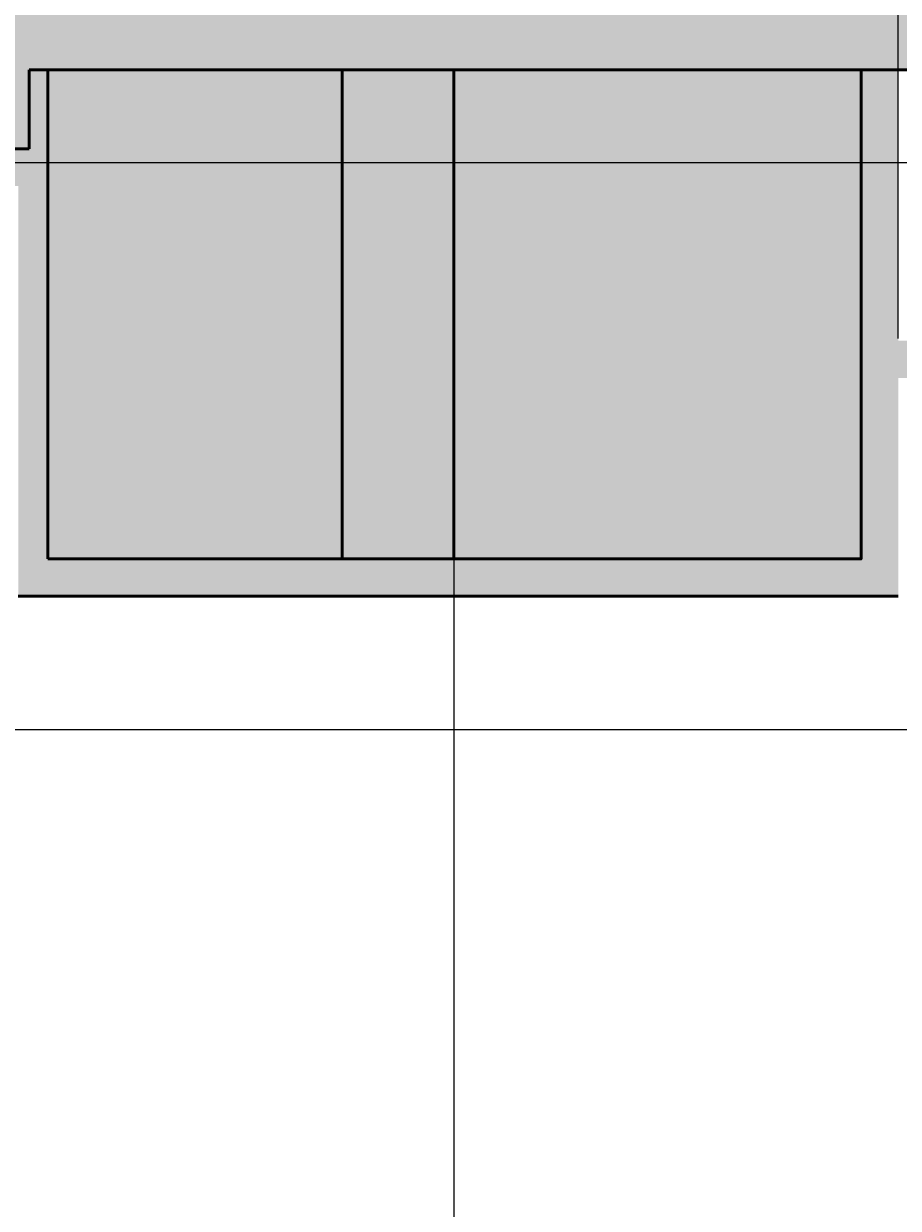
# Model space of a CAD drawing. Units: inches. Extents: x -12 to 334, y -10 to 186.
# Tile 13 of 77: x 64 to 88, y 33 to 65. Entities that reach past the tile are written whole.
import ezdxf
from ezdxf import colors
from ezdxf.entities.mleader import LeaderData, LeaderLine
from ezdxf.math import Vec2, Vec3

# ---------------------------------------------------------------- set-up
doc = ezdxf.new("R2010")
doc.units = ezdxf.units.IN
doc.header["$MEASUREMENT"] = 0
for name, color, linetype, lineweight in [('M-ANNO-TEXT', 3, 'Continuous', 25), ('M-DIMS', 2, 'Continuous', 18), ('M-EQPM', 7, 'Continuous', 50), ('M-EQPM-PATT', 8, 'Continuous', 18)]:
    doc.layers.add(name, color=color, linetype=linetype, lineweight=lineweight)
doc.styles.get("Standard").update_dxf_attribs({"font": 'arial.ttf'})
doc.dimstyles.get("Standard").update_dxf_attribs({"dimtxt": 0.18, "dimasz": 0.18, "dimexe": 0.18, "dimexo": 0.0625, "dimgap": 0.09, "dimtad": 0, "dimtih": 1, "dimtoh": 1, "dimdec": 4, "dimzin": 0, "dimdsep": 46, "dimtxsty": 'Standard', "dimcen": 0.09, "dimadec": 0, "dimazin": 0, "dimtfac": 1, "dimtdec": 4, "dimtofl": 0, "dimtmove": 0, "dimatfit": 3, "dimfxl": 1, "dimtolj": 1, "dimtzin": 0, "dimarcsym": 0})

# ---------------------------------------------------------------- blocks, each defined once
blk = doc.blocks.new('*D1')
at = {"layer": 'Defpoints', "color": 0, "transparency": 16777216}
for p in [(281.426, 91.899), (3.376, 80.692), (281.426, 14.304)]:
    blk.add_point(p, dxfattribs=at)
at = {"layer": 'M-DIMS', "color": 0, "lineweight": -2, "transparency": 16777216}
for p, q in [((281.426, 91.836), (281.426, 14.124)), ((3.376, 80.629), (3.376, 14.124)), ((3.556, 14.304), (141.935, 14.304)), ((281.246, 14.304), (142.867, 14.304))]:
    blk.add_line(p, q, dxfattribs=at)
at = {"layer": 'M-DIMS', "color": 0, "transparency": 16777216}
for points in [[(3.556, 14.334), (3.556, 14.274), (3.376, 14.304)], [(281.246, 14.334), (281.246, 14.274), (281.426, 14.304)]]:
    blk.add_solid(points, dxfattribs=at)
at = {"layer": 'M-DIMS', "color": 0, "transparency": 16777216, "insert": (142.401, 14.304), "char_height": 0.18, "attachment_point": 5}
blk.add_mtext('\\A1;278.05', dxfattribs=at)
blk = doc.blocks.new('*D26')
at = {"layer": 'Defpoints', "color": 0, "transparency": 16777216}
for p in [(87.888, 169.385), (87.888, 56.321), (58.1, 33.675)]:
    blk.add_point(p, dxfattribs=at)
at = {"layer": 'M-DIMS', "color": 0, "lineweight": -2, "transparency": 16777216}
for p, q in [((58.1, 33.738), (58.1, 169.565)), ((58.28, 169.385), (72.599, 169.385)), ((87.708, 169.385), (73.389, 169.385)), ((87.888, 56.383), (87.888, 169.565))]:
    blk.add_line(p, q, dxfattribs=at)
at = {"layer": 'M-DIMS', "color": 0, "transparency": 16777216}
for points in [[(58.28, 169.415), (58.28, 169.355), (58.1, 169.385)], [(87.708, 169.415), (87.708, 169.355), (87.888, 169.385)]]:
    blk.add_solid(points, dxfattribs=at)
at = {"layer": 'M-DIMS', "color": 0, "transparency": 16777216, "insert": (72.994, 169.385), "char_height": 0.18, "attachment_point": 5}
blk.add_mtext('\\A1;29.79', dxfattribs=at)
blk = doc.blocks.new('*D29')
at = {"layer": 'Defpoints', "color": 0, "transparency": 16777216}
for p in [(-11.174, 45.854), (221.576, 45.854), (216.576, 30.854)]:
    blk.add_point(p, dxfattribs=at)
at = {"layer": 'M-DIMS', "color": 0, "lineweight": -2, "transparency": 16777216}
for p, q in [((221.514, 45.854), (-11.354, 45.854)), ((-11.174, 45.674), (-11.174, 38.536)), ((-11.174, 31.034), (-11.174, 38.172)), ((216.514, 30.854), (-11.354, 30.854))]:
    blk.add_line(p, q, dxfattribs=at)
at = {"layer": 'M-DIMS', "color": 0, "transparency": 16777216}
for points in [[(-11.204, 45.674), (-11.144, 45.674), (-11.174, 45.854)], [(-11.204, 31.034), (-11.144, 31.034), (-11.174, 30.854)]]:
    blk.add_solid(points, dxfattribs=at)
at = {"layer": 'M-DIMS', "color": 0, "transparency": 16777216, "insert": (-11.174, 38.354), "char_height": 0.18, "attachment_point": 5}
blk.add_mtext('\\A1;15', dxfattribs=at)
blk = doc.blocks.new('*D30')
at = {"layer": 'Defpoints', "color": 0, "transparency": 16777216}
for p in [(75.924, 63.612), (129.093, 61.105), (129.093, 14.304)]:
    blk.add_point(p, dxfattribs=at)
at = {"layer": 'M-DIMS', "color": 0, "lineweight": -2, "transparency": 16777216}
for p, q in [((75.924, 63.549), (75.924, 14.124)), ((129.093, 61.042), (129.093, 14.124)), ((76.104, 14.304), (102.115, 14.304)), ((128.913, 14.304), (102.902, 14.304))]:
    blk.add_line(p, q, dxfattribs=at)
at = {"layer": 'M-DIMS', "color": 0, "transparency": 16777216}
for points in [[(76.104, 14.334), (76.104, 14.274), (75.924, 14.304)], [(128.913, 14.334), (128.913, 14.274), (129.093, 14.304)]]:
    blk.add_solid(points, dxfattribs=at)
at = {"layer": 'M-DIMS', "color": 0, "transparency": 16777216, "insert": (102.509, 14.304), "char_height": 0.18, "attachment_point": 5}
blk.add_mtext('\\A1;53.17', dxfattribs=at)
blk = doc.blocks.new('*D35')
at = {"layer": 'Defpoints', "color": 0, "transparency": 16777216}
for p in [(216.428, 98.108), (-11.174, 61.105), (216.428, 61.105)]:
    blk.add_point(p, dxfattribs=at)
at = {"layer": 'M-DIMS', "color": 0, "lineweight": -2, "transparency": 16777216}
for p, q in [((216.365, 98.108), (-11.354, 98.108)), ((-11.174, 97.928), (-11.174, 79.788)), ((-11.174, 61.285), (-11.174, 79.424)), ((216.365, 61.105), (-11.354, 61.105))]:
    blk.add_line(p, q, dxfattribs=at)
at = {"layer": 'M-DIMS', "color": 0, "transparency": 16777216}
for points in [[(-11.204, 97.928), (-11.144, 97.928), (-11.174, 98.108)], [(-11.204, 61.285), (-11.144, 61.285), (-11.174, 61.105)]]:
    blk.add_solid(points, dxfattribs=at)
at = {"layer": 'M-DIMS', "color": 0, "transparency": 16777216, "insert": (-11.174, 79.606), "char_height": 0.18, "attachment_point": 5}
blk.add_mtext('\\A1;37', dxfattribs=at)
blk = doc.blocks.new('*D39')
at = {"layer": 'Defpoints', "color": 0, "transparency": 16777216}
for p in [(279.726, 80.692), (-11.174, 45.854), (269.381, 45.854)]:
    blk.add_point(p, dxfattribs=at)
at = {"layer": 'M-DIMS', "color": 0, "lineweight": -2, "transparency": 16777216}
for p, q in [((279.664, 80.692), (-11.354, 80.692)), ((-11.174, 80.512), (-11.174, 63.455)), ((-11.174, 46.034), (-11.174, 63.091)), ((269.318, 45.854), (-11.354, 45.854))]:
    blk.add_line(p, q, dxfattribs=at)
at = {"layer": 'M-DIMS', "color": 0, "transparency": 16777216}
for points in [[(-11.204, 80.512), (-11.144, 80.512), (-11.174, 80.692)], [(-11.204, 46.034), (-11.144, 46.034), (-11.174, 45.854)]]:
    blk.add_solid(points, dxfattribs=at)
at = {"layer": 'M-DIMS', "color": 0, "transparency": 16777216, "insert": (-11.174, 63.273), "char_height": 0.18, "attachment_point": 5}
blk.add_mtext('\\A1;34.84', dxfattribs=at)

msp = doc.modelspace()

# ---------------------------------------------------------------- hatches: boundary and pattern name
at = {"layer": 'M-EQPM-PATT'}
h = msp.add_hatch(color=256, dxfattribs=at)
h.set_gradient(color1=(99, 100, 102), color2=(99, 100, 102), tint=1)
h.paths.add_polyline_path([(4.3766, 80.754, -0.4132606), (23.5807, 99.8958), (37.1002, 99.8958), (37.1002, 127.7078), (32.1002, 127.7078), (32.1002, 125.2078), (36.1002, 125.2078), (36.1002, 100.8958), (23.5807, 100.8958, 1), (23.5807, 60.4872), (36.1002, 60.4872), (36.1002, 36.1752), (32.1002, 36.1752), (32.1002, 33.6752), (37.1002, 33.6752), (37.1002, 61.4872), (23.5807, 61.4872, -0.384914), (4.4744, 78.754), (72.9244, 78.754), (72.9244, 69.6117), (75.9244, 69.6117), (75.9244, 89.8963), (72.9244, 89.8963), (72.9244, 80.754)])
h.paths.add_polyline_path([(54.1002, 125.2078), (58.1002, 125.2078), (58.1002, 127.7078), (53.1002, 127.7078), (53.1002, 99.8958), (64.5, 99.8958), (64.5, 109.0583), (63.5, 109.0583), (63.5, 100.8958), (54.1002, 100.8958)], flags=17)
h.paths.add_polyline_path([(53.1002, 33.6752), (58.1002, 33.6752), (58.1002, 36.1752), (54.1002, 36.1752), (54.1002, 60.4872), (64.2068, 60.4872), (64.2068, 49.4497), (87.8879, 49.4497), (87.8879, 55.3205), (104.8919, 55.3205), (104.8919, 30.8541), (99.8919, 30.8541), (99.8919, 28.8541), (105.8919, 28.8541), (105.8919, 56.3205), (87.8879, 56.3205), (87.8879, 63.6117), (86.8879, 63.6117), (86.8879, 50.4497), (65.0061, 50.4497), (65.0061, 63.6117), (64.5, 63.6117), (64.5, 61.4872), (53.1002, 61.4872)])
h.paths.add_polyline_path([(121.8919, 28.8541), (121.8919, 30.8541), (116.8919, 30.8541), (116.8919, 45.8541), (209.6965, 45.8541), (209.9204, 46.8541), (115.8919, 46.8541), (115.8919, 28.8541)])
h.paths.add_polyline_path([(221.5761, 32.8541), (216.5761, 32.8541), (216.5761, 30.8541), (222.5761, 30.8541), (222.5761, 46.8541), (209.9204, 46.8541), (209.6965, 45.8541), (221.5761, 45.8541)])
h.paths.add_polyline_path([(233.5761, 45.8541), (249.8485, 45.8541), (249.3759, 46.8541), (232.5761, 46.8541), (232.5761, 30.8541), (238.5761, 30.8541), (238.5761, 32.8541), (233.5761, 32.8541)])
h = msp.add_hatch(color=256, dxfattribs=at)
h.set_gradient(color1=(205, 32, 39), color2=(205, 32, 39), tint=1)
h.paths.add_polyline_path([(64.5, 80.754), (64.5, 89.8963), (226.6083, 89.8963, -1), (226.6083, 69.6117), (64.5, 69.6117), (64.5, 78.754), (4.4744, 78.754, 0.384914), (23.5807, 61.4872), (37.1002, 61.4872), (37.1002, 33.6752), (53.1002, 33.6752), (53.1002, 61.4872), (64.5, 61.4872), (64.5, 63.6117), (226.6083, 63.6117, 1), (226.6083, 95.8963), (64.5, 95.8963), (64.5, 99.8958), (53.1002, 99.8958), (53.1002, 127.7078), (37.1002, 127.7078), (37.1002, 99.8958), (23.5807, 99.8958, 0.4132606), (4.3766, 80.754)])
h.paths.add_polyline_path([(64.5, 91.8963), (64.5, 93.8963), (226.6083, 93.8963, -1), (226.6083, 65.6117), (64.5, 65.6117), (64.5, 67.6117), (226.6083, 67.6117, 1), (226.6083, 91.8963)], flags=16)
h = msp.add_hatch(color=256, dxfattribs=at)
h.set_gradient(color1=(205, 32, 39), color2=(205, 32, 39), tint=1)
h.paths.add_polyline_path([(72.9244, 95.8963), (72.9244, 109.0583), (64.5, 109.0583), (64.5, 95.8963)])
h.paths.add_polyline_path([(72.9244, 80.754), (72.9244, 89.8963), (64.5, 89.8963), (64.5, 80.754)])
h.paths.add_polyline_path([(72.9244, 69.6117), (72.9244, 78.754), (64.5, 78.754), (64.5, 69.6117)])
h.paths.add_polyline_path([(72.9244, 50.4497), (72.9244, 63.6117), (65.0061, 63.6117), (65.0061, 50.4497)])
h = msp.add_hatch(color=256, dxfattribs=at)
h.set_gradient(color1=(99, 100, 102), color2=(99, 100, 102), tint=1)
h.paths.add_polyline_path([(72.9244, 95.8963), (75.9244, 95.8963), (75.9244, 109.0583), (72.9244, 109.0583)])
h.paths.add_polyline_path([(72.9244, 50.4497), (75.9244, 50.4497), (75.9244, 63.6117), (72.9244, 63.6117)])
h.paths.add_polyline_path([(75.9244, 91.8963), (75.9244, 93.8963), (72.9244, 93.8963), (72.9244, 91.8963)])
h.paths.add_polyline_path([(75.9244, 65.6117), (75.9244, 67.6117), (72.9244, 67.6117), (72.9244, 65.6117)])
h.paths.add_polyline_path([(129.093, 69.6117), (130.8573, 69.6117), (130.8573, 89.8963), (129.093, 89.8963)])
h.paths.add_polyline_path([(129.093, 98.1081), (129.093, 95.8963), (130.8573, 95.8963), (130.8573, 98.1081)])
h.paths.add_polyline_path([(130.8573, 61.1045), (130.8573, 63.6117), (129.093, 63.6117), (129.093, 61.1045)])
h.paths.add_polyline_path([(170.9079, 69.6117), (172.6722, 69.6117), (172.6722, 89.8963), (170.9079, 89.8963)])
h.paths.add_polyline_path([(172.6722, 95.8963), (172.6722, 98.1081), (170.9079, 98.1081), (170.9079, 95.8963)])
h.paths.add_polyline_path([(170.9079, 61.1045), (172.6722, 61.1045), (172.6722, 63.6117), (170.9079, 63.6117)])
h.paths.add_polyline_path([(218.1922, 63.6117), (216.4278, 63.6117), (216.4278, 61.1045), (218.1922, 61.1045)])
h.paths.add_polyline_path([(216.4278, 69.6117), (218.1922, 69.6117), (218.1922, 89.8963), (216.4278, 89.8963)])
h.paths.add_polyline_path([(216.4278, 95.8963), (218.1922, 95.8963), (218.1922, 98.1081), (216.4278, 98.1081)])
h = msp.add_hatch(color=256, dxfattribs=at)
h.set_gradient(color1=(94, 103, 175), color2=(94, 103, 175), tint=1)
h.paths.add_polyline_path([(86.8879, 50.4497), (86.8879, 63.6117), (75.9244, 63.6117), (75.9244, 50.4497)])

# ---------------------------------------------------------------- linework, layer by layer
at = {"layer": 'M-EQPM'}
for p, q in [((65.0061, 63.6117), (65.0061, 50.4497)), ((72.9244, 63.6117), (72.9244, 50.4497)), ((75.9244, 63.6117), (75.9244, 50.4497)), ((87.8879, 49.4497), (64.2068, 49.4497))]:
    msp.add_line(p, q, dxfattribs=at)
msp.add_lwpolyline([(64.5, 63.6117), (226.6083, 63.6117, 1), (226.6083, 95.8963), (64.5, 95.8963)], format="xyb", dxfattribs=at)
for points in [[(64.5, 61.4872), (64.5, 63.6117)], [(86.8879, 63.6117), (86.8879, 50.4497), (65.0061, 50.4497)], [(64.5, 61.4872), (53.1002, 61.4872)]]:
    msp.add_lwpolyline(points, dxfattribs=at)

# ---------------------------------------------------------------- dimensions: what is measured, and where the dimension line sits
at = {"layer": 'M-DIMS'}
for base, p1, p2, picture, middle in [((87.8879, 169.3845), (58.1002, 33.6752), (87.8879, 56.3205), '*D26', (72.9941, 169.3845)), ((281.4256, 14.3041), (3.3765, 80.6915), (281.4256, 91.8988), '*D1', (142.401, 14.3041)), ((129.093, 14.3041), (75.9244, 63.6117), (129.093, 61.1045), '*D30', (102.5087, 14.3041))]:
    dim = msp.add_linear_dim(base=base, p1=p1, p2=p2, dimstyle='Standard', override={"dimdec": 2, "dimlfac": 1, "dimrnd": 0, "dimzin": 0, "dimdsep": 46, "dimlunit": 2}, dxfattribs=at)
    dim.commit()
    dim.dimension.update_dxf_attribs({"geometry": picture, "text_midpoint": middle})
for base, p1, p2, override, picture, middle in [((-11.1736, 61.1045), (216.4278, 98.1081), (216.4278, 61.1045), {"dimdec": 0, "dimlfac": 1, "dimrnd": 0, "dimzin": 0, "dimdsep": 46, "dimlunit": 2}, '*D35', (-11.1735, 79.6063)), ((-11.1736, 45.8541), (279.7263, 80.6915), (269.3808, 45.8541), {"dimdec": 2, "dimlfac": 1, "dimrnd": 0, "dimzin": 0, "dimdsep": 46, "dimlunit": 2}, '*D39', (-11.1735, 63.2728)), ((-11.1736, 45.8541), (216.5761, 30.8541), (221.5761, 45.8541), {"dimdec": 0, "dimlfac": 1, "dimrnd": 0, "dimzin": 0, "dimdsep": 46, "dimlunit": 2}, '*D29', (-11.1735, 38.3541))]:
    dim = msp.add_linear_dim(base=base, p1=p1, p2=p2, angle=90, dimstyle='Standard', override=override, dxfattribs=at)
    dim.commit()
    dim.dimension.update_dxf_attribs({"geometry": picture, "text_midpoint": middle})

# ---------------------------------------------------------------- leaders
at = {"layer": 'M-ANNO-TEXT'}
ml = msp.add_multileader_mtext('Standard', dxfattribs=at)
ml.set_content('^ICondensate outlet', color=256)
ml.set_leader_properties()
ml.build(insert=Vec2(0, 0))
ml.multileader.update_dxf_attribs({"dogleg_length": 0.36, "arrow_head_size": 0.7})
ctx = ml.context
ctx.base_point, ctx.arrow_head_size, ctx.landing_gap_size, ctx.plane_origin = Vec3(83.8784, 10.3512), 0.7, 0.09, Vec3(49.4251, 25.7584)
notes = []
notes.append((ctx, [(0, (1, 1, 0), (70.8242, 10.3512), (1, 0), 13.0542, [(0, [(42.9275, 33.6752)], 0, [])])]))
ctx.mtext.insert, ctx.mtext.flow_direction = Vec3(83.9684, 12.3853), 5
for ctx, leaders in notes:
    for number, flags, end, landing, length, lines in leaders:
        leader = LeaderData()
        leader.index, (leader.has_last_leader_line, leader.has_dogleg_vector, leader.attachment_direction) = number, flags
        leader.last_leader_point, leader.dogleg_vector, leader.dogleg_length = Vec3(end), Vec3(landing), length
        for number, points, colour, breaks in lines:
            line = LeaderLine()
            line.index, line.vertices, line.color, line.breaks = number, Vec3.list(points), colors.encode_raw_color(colour), breaks
            leader.lines.append(line)
        ctx.leaders.append(leader)

doc.saveas('drawing.dxf')
